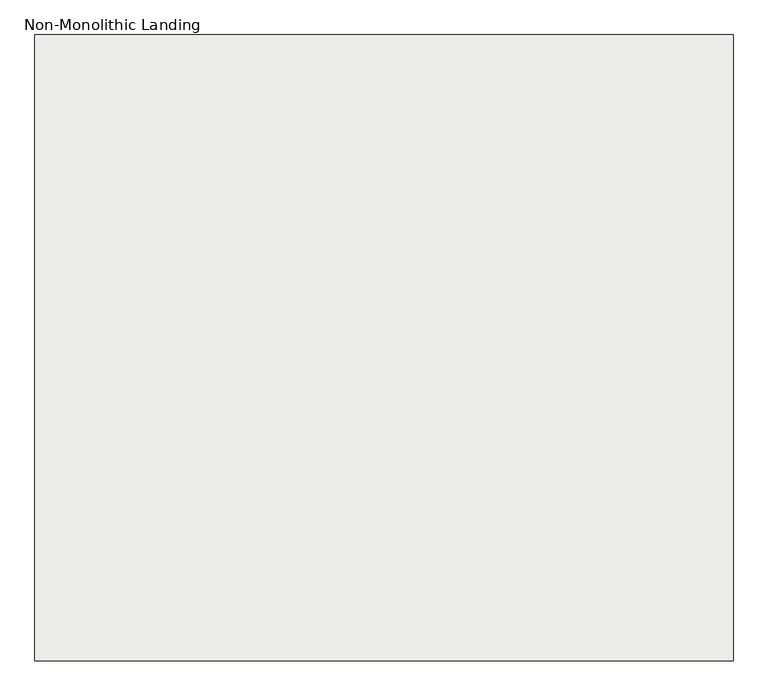
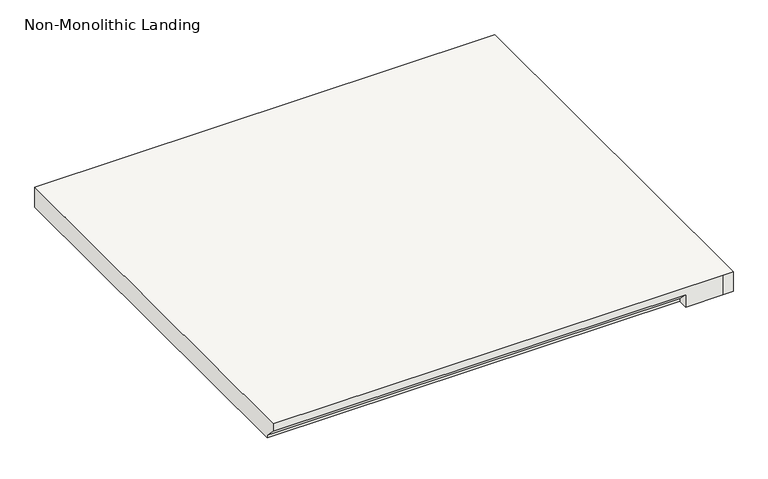
"""IFC4 building model written with IfcOpenShell, lengths in millimetres: slab geometry, Non-Monolithic Landing."""

from ifc_helpers import new_model, si_unit, origin, place, context, project, spatial, faceted_brep, source, transform, mapped, element, save


def non_monolithic_landing_3e227109(model_context):
    return source(origin(), model_context, "Body", "Brep", [
        faceted_brep([(-7815.6002526, 11195.5128362, 1200.15), (-7815.6002526, 11220.9128362, 1174.75), (-6818.6502526, 11220.9128362, 1174.75), (-6818.6502526, 11195.5128362, 1200.15), (-6729.7502524, 11195.5128362, 1219.2), (-6704.3502524, 11195.5128362, 1219.2), (-6704.3502524, 12192.4628362, 1219.2), (-6729.7502524, 12192.4628362, 1219.2), (-7815.6002526, 12192.4628362, 1219.2), (-7815.6002526, 11195.5128362, 1219.2), (-6818.6502526, 11220.9128362, 1168.4), (-7815.6002526, 11220.9128362, 1168.4), (-7815.6002526, 12192.4628362, 1168.4), (-6729.7502524, 12192.4628362, 1168.4), (-6704.3502524, 12192.4628362, 1168.4), (-6704.3502524, 11195.5128362, 1168.4), (-6729.7502524, 11195.5128362, 1168.4), (-6818.6502526, 11195.5128362, 1168.4)], [[[0, 1, 2, 3]], [[4, 5, 6, 7, 8, 9]], [[10, 11, 12, 13, 14, 15, 16, 17]], [[11, 10, 2, 1]], [[10, 17, 3, 2]], [[4, 9, 0, 3, 17, 16]], [[5, 4, 16, 15]], [[6, 5, 15, 14]], [[7, 6, 14, 13]], [[8, 7, 13, 12]], [[9, 8, 12, 11, 1, 0]]]),
    ])


if __name__ == "__main__":
    model = new_model("IFC4")
    model_context = context("Model", 3, world=origin())
    ifc_project = project(units=[si_unit("LENGTHUNIT", "METRE", prefix="MILLI")], contexts=[model_context])
    site = spatial("IfcSite", under=ifc_project)
    building = spatial("IfcBuilding", under=site)
    placement = place(None, origin())
    non_monolithic_landing_shape = non_monolithic_landing_3e227109(model_context)
    element("IfcSlab", 1, ObjectType="Non-Monolithic Landing", at=placement, inside=building, context=model_context, shape_type="MappedRepresentation", body=[
        mapped(non_monolithic_landing_shape, transform((0.0, 0.0, 0.0), x_axis=(1.0, 0.0, 0.0), y_axis=(0.0, 1.0, 0.0), z_axis=(0.0, 0.0, 1.0))),
    ])
    save(model, "model.ifc")
